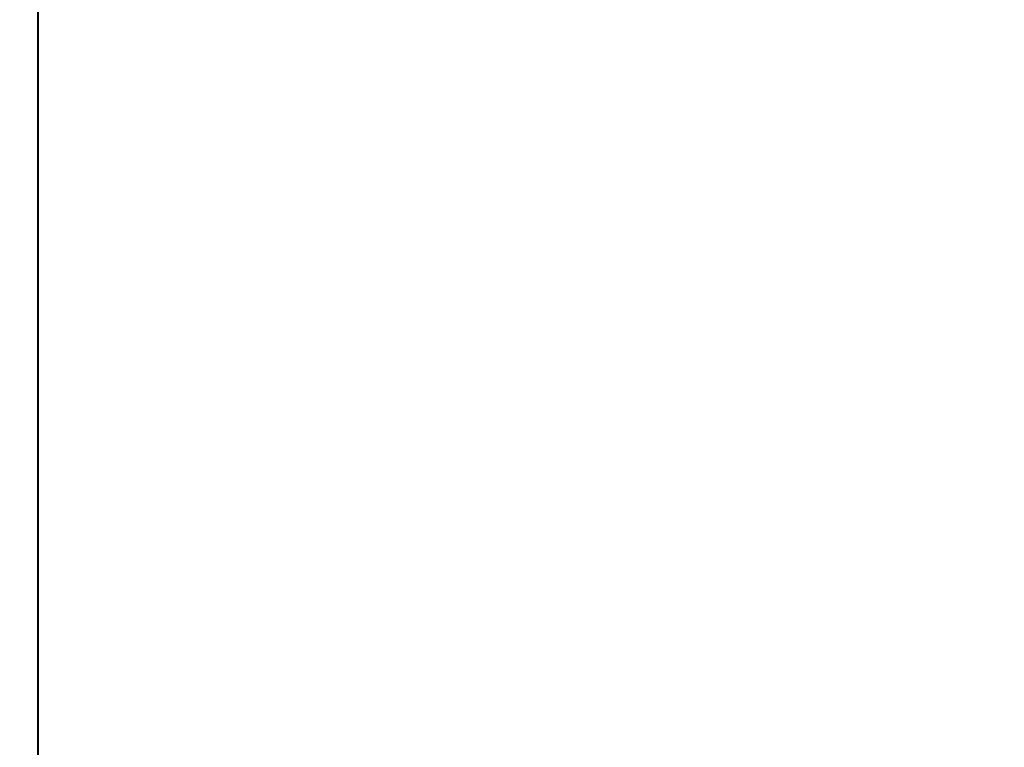
# Model space of a CAD drawing. Units: inches. Extents: x 459864 to 460310, y 324185 to 324787.
# Tile 95 of 112: x 460247.1043 to 460247.6764, y 324283.8523 to 324284.2752. Entities that reach past the tile are written whole.
import ezdxf

# ---------------------------------------------------------------- set-up
doc = ezdxf.new("R2010")
doc.units = ezdxf.units.IN
doc.layers.add('A-ANNO-DIMS', color=2, linetype='Continuous', lineweight=18)
doc.layers.add('A-WALL', color=7, linetype='Continuous', lineweight=40)
doc.styles.get("Standard").update_dxf_attribs({"font": 'arial.ttf'})
doc.dimstyles.new('ISO-25', dxfattribs={"dimtxt": 6, "dimasz": 2.5, "dimexe": 1.25, "dimexo": 0.625, "dimtad": 1, "dimdec": 1, "dimlunit": 3, "dimtxsty": 'Standard', "dimcen": 2.5, "dimadec": 0, "dimazin": 0, "dimtfac": 1, "dimtdec": 1, "dimtmove": 0, "dimatfit": 3, "dimfxl": 1, "dimarcsym": 0})

# ---------------------------------------------------------------- blocks, each defined once
blk = doc.blocks.new('*D21')
at = {"layer": 'A-ANNO-DIMS', "color": 0, "lineweight": -2, "transparency": 16777216}
for p, q in [((460247.73993, 324715.48323), (460309.58037, 324715.48323)), ((460308.33037, 324712.98323), (460308.33037, 324285.98323)), ((460247.73993, 324283.48323), (460309.58037, 324283.48323))]:
    blk.add_line(p, q, dxfattribs=at)
at = {"layer": 'A-ANNO-DIMS', "color": 0, "transparency": 16777216}
for points in [[(460307.9137, 324712.98323), (460308.74704, 324712.98323), (460308.33037, 324715.48323)], [(460307.9137, 324285.98323), (460308.74704, 324285.98323), (460308.33037, 324283.48323)]]:
    blk.add_solid(points, dxfattribs=at)
at = {"layer": 'Defpoints', "color": 0, "transparency": 16777216}
for p in [(460247.11493, 324715.48323), (460247.11493, 324283.48323), (460308.33037, 324283.48323)]:
    blk.add_point(p, dxfattribs=at)
at = {"layer": 'A-ANNO-DIMS', "color": 0, "transparency": 16777216, "insert": (460304.63988, 324499.48323), "char_height": 6, "attachment_point": 5, "rotation": 90}
blk.add_mtext("36'", dxfattribs=at)
blk = doc.blocks.new('*D62')
at = {"layer": 'A-ANNO-DIMS', "color": 0, "lineweight": -2, "transparency": 16777216}
for p, q in [((460247.73993, 324332.73872), (460278.76493, 324332.73872)), ((460277.51493, 324330.23872), (460277.51493, 324285.98323)), ((460247.73993, 324283.48323), (460278.76493, 324283.48323))]:
    blk.add_line(p, q, dxfattribs=at)
at = {"layer": 'A-ANNO-DIMS', "color": 0, "transparency": 16777216}
for points in [[(460277.09826, 324330.23872), (460277.93159, 324330.23872), (460277.51493, 324332.73872)], [(460277.09826, 324285.98323), (460277.93159, 324285.98323), (460277.51493, 324283.48323)]]:
    blk.add_solid(points, dxfattribs=at)
at = {"layer": 'Defpoints', "color": 0, "transparency": 16777216}
for p in [(460247.11493, 324332.73872), (460247.11493, 324283.48323), (460277.51493, 324283.48323)]:
    blk.add_point(p, dxfattribs=at)
at = {"layer": 'A-ANNO-DIMS', "color": 0, "transparency": 16777216, "insert": (460273.78761, 324308.11098), "char_height": 6, "attachment_point": 5, "rotation": 90}
blk.add_mtext('4\'-1 1/2"', dxfattribs=at)
blk = doc.blocks.new('*D67')
at = {"layer": 'A-ANNO-DIMS', "color": 0, "lineweight": -2, "transparency": 16777216}
for p, q in [((460208.11493, 324284.10823), (460208.11493, 324315.13323)), ((460247.11493, 324284.10823), (460247.11493, 324315.13323)), ((460210.61493, 324313.88323), (460244.61493, 324313.88323))]:
    blk.add_line(p, q, dxfattribs=at)
at = {"layer": 'A-ANNO-DIMS', "color": 0, "transparency": 16777216}
for points in [[(460210.61493, 324314.2999), (460210.61493, 324313.46657), (460208.11493, 324313.88323)], [(460244.61493, 324314.2999), (460244.61493, 324313.46657), (460247.11493, 324313.88323)]]:
    blk.add_solid(points, dxfattribs=at)
at = {"layer": 'Defpoints', "color": 0, "transparency": 16777216}
for p in [(460247.11493, 324313.88323), (460208.11493, 324283.48323), (460247.11493, 324283.48323)]:
    blk.add_point(p, dxfattribs=at)
at = {"layer": 'A-ANNO-DIMS', "color": 0, "transparency": 16777216, "insert": (460227.61493, 324317.57372), "char_height": 6, "attachment_point": 5}
blk.add_mtext('3\'-3"', dxfattribs=at)

msp = doc.modelspace()

# ---------------------------------------------------------------- linework, layer by layer
at = {"layer": 'A-WALL'}
msp.add_line((460247.11493, 324470.98323), (460247.11493, 324283.48323), dxfattribs=at)

# ---------------------------------------------------------------- dimensions: what is measured, and where the dimension line sits
at = {"layer": 'A-ANNO-DIMS'}
for base, p1, angle, override, picture, middle in [((460308.33037, 324283.48323), (460247.11493, 324715.48323), 90, {"dimclrd": 0, "dimclre": 0, "dimclrt": 0}, '*D21', (460304.63988, 324499.48323)), ((460277.51493, 324283.48323), (460247.11493, 324332.73872), 270, {"dimdec": 1, "dimlfac": 1, "dimrnd": 0, "dimzin": 1, "dimdsep": 46, "dimlunit": 4, "dimfrac": 2}, '*D62', (460273.78761, 324308.11098))]:
    dim = msp.add_linear_dim(base=base, p1=p1, p2=(460247.11493, 324283.48323), angle=angle, dimstyle='ISO-25', override=override, dxfattribs=at)
    dim.commit()
    dim.dimension.update_dxf_attribs({"geometry": picture, "text_midpoint": middle})
dim = msp.add_linear_dim(base=(460247.11493, 324313.88323), p1=(460208.11493, 324283.48323), p2=(460247.11493, 324283.48323), dimstyle='ISO-25', override={"dimdec": 1, "dimlfac": 1, "dimrnd": 0, "dimzin": 1, "dimdsep": 46, "dimlunit": 4, "dimfrac": 2}, dxfattribs=at)
dim.commit()
dim.dimension.update_dxf_attribs({"geometry": '*D67', "text_midpoint": (460227.61493, 324317.57372)})

doc.saveas('drawing.dxf')
